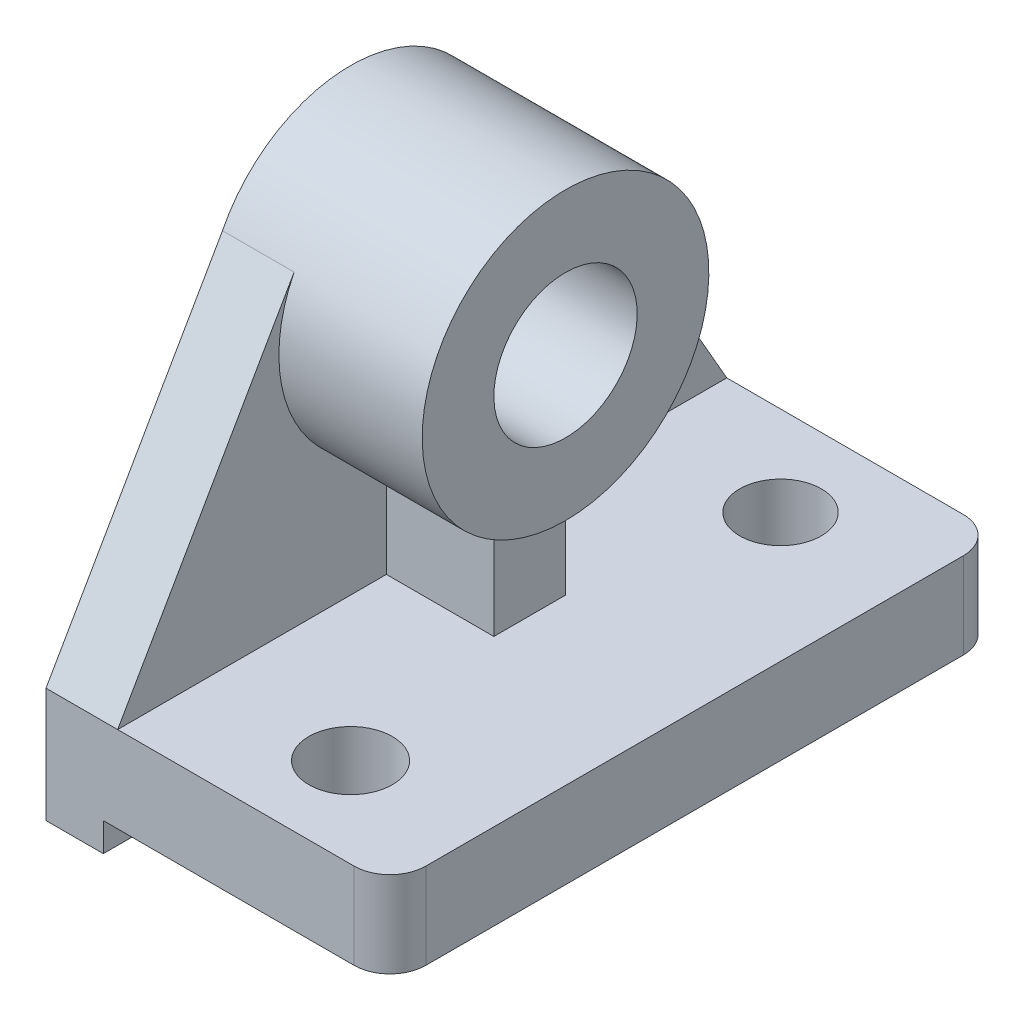
ISO-10303-21;
HEADER;
FILE_DESCRIPTION(('STEP AP214'),'2;1');
FILE_NAME('part.step','',(''),(''),'','','');
FILE_SCHEMA(('AUTOMOTIVE_DESIGN { 1 0 10303 214 1 1 1 1 }'));
ENDSEC;
DATA;
#1=APPLICATION_CONTEXT('core data for automotive mechanical design processes');
#2=APPLICATION_PROTOCOL_DEFINITION('international standard','automotive_design',2000,#1);
#3=PRODUCT_CONTEXT('',#1,'mechanical');
#4=PRODUCT('Part','Part','',(#3));
#5=PRODUCT_RELATED_PRODUCT_CATEGORY('part','',(#4));
#6=PRODUCT_DEFINITION_FORMATION('','',#4);
#7=PRODUCT_DEFINITION_CONTEXT('part definition',#1,'design');
#8=PRODUCT_DEFINITION('design','',#6,#7);
#9=PRODUCT_DEFINITION_SHAPE('','',#8);
#10=(LENGTH_UNIT() NAMED_UNIT(*) SI_UNIT(.MILLI.,.METRE.));
#11=(NAMED_UNIT(*) PLANE_ANGLE_UNIT() SI_UNIT($,.RADIAN.));
#12=(NAMED_UNIT(*) SI_UNIT($,.STERADIAN.) SOLID_ANGLE_UNIT());
#13=UNCERTAINTY_MEASURE_WITH_UNIT(LENGTH_MEASURE(1.E-05),#10,'distance_accuracy_value','');
#14=(GEOMETRIC_REPRESENTATION_CONTEXT(3) GLOBAL_UNCERTAINTY_ASSIGNED_CONTEXT((#13)) GLOBAL_UNIT_ASSIGNED_CONTEXT((#10,
#11,#12)) REPRESENTATION_CONTEXT('',''));
#15=CARTESIAN_POINT('',(0.,0.,0.));
#16=DIRECTION('',(0.,0.,1.));
#17=DIRECTION('',(1.,0.,0.));
#18=AXIS2_PLACEMENT_3D('',#15,#16,#17);
#19=CARTESIAN_POINT('',(0.,16.,85.));
#20=DIRECTION('',(0.,-1.,0.));
#21=DIRECTION('',(1.,0.,0.));
#22=AXIS2_PLACEMENT_3D('',#19,#20,#21);
#23=PLANE('',#22);
#24=CARTESIAN_POINT('',(30.,16.,12.5));
#25=DIRECTION('',(0.,1.,0.));
#26=DIRECTION('',(-1.,0.,0.));
#27=AXIS2_PLACEMENT_3D('',#24,#25,#26);
#28=CIRCLE('',#27,5.6970542524879);
#29=CARTESIAN_POINT('',(24.3029457475121,16.,12.5));
#30=VERTEX_POINT('',#29);
#31=EDGE_CURVE('E251',#30,#30,#28,.T.);
#32=ORIENTED_EDGE('',*,*,#31,.F.);
#33=EDGE_LOOP('',(#32));
#34=FACE_BOUND('',#33,.T.);
#35=CARTESIAN_POINT('',(30.,16.,72.5));
#36=DIRECTION('',(0.,1.,0.));
#37=DIRECTION('',(-1.,0.,0.));
#38=AXIS2_PLACEMENT_3D('',#35,#36,#37);
#39=CIRCLE('',#38,5.82954388626669);
#40=CARTESIAN_POINT('',(24.1704561137333,16.,72.5));
#41=VERTEX_POINT('',#40);
#42=EDGE_CURVE('E314',#41,#41,#39,.T.);
#43=ORIENTED_EDGE('',*,*,#42,.F.);
#44=EDGE_LOOP('',(#43));
#45=FACE_BOUND('',#44,.T.);
#46=DIRECTION('',(0.,0.,-1.));
#47=VECTOR('',#46,1.);
#48=CARTESIAN_POINT('',(48.,16.,85.));
#49=LINE('',#48,#47);
#50=CARTESIAN_POINT('',(48.,16.,80.));
#51=VERTEX_POINT('',#50);
#52=CARTESIAN_POINT('',(48.,16.,5.));
#53=VERTEX_POINT('',#52);
#54=EDGE_CURVE('E238',#51,#53,#49,.T.);
#55=ORIENTED_EDGE('',*,*,#54,.T.);
#56=CARTESIAN_POINT('',(43.,16.,5.));
#57=DIRECTION('',(0.,-1.,0.));
#58=DIRECTION('',(1.,0.,0.));
#59=AXIS2_PLACEMENT_3D('',#56,#57,#58);
#60=CIRCLE('',#59,5.);
#61=CARTESIAN_POINT('',(43.,16.,0.));
#62=VERTEX_POINT('',#61);
#63=EDGE_CURVE('E265',#53,#62,#60,.F.);
#64=ORIENTED_EDGE('',*,*,#63,.T.);
#65=DIRECTION('',(-1.,0.,0.));
#66=VECTOR('',#65,1.);
#67=CARTESIAN_POINT('',(0.,16.,0.));
#68=LINE('',#67,#66);
#69=CARTESIAN_POINT('',(10.,16.,0.));
#70=VERTEX_POINT('',#69);
#71=EDGE_CURVE('E231',#62,#70,#68,.T.);
#72=ORIENTED_EDGE('',*,*,#71,.T.);
#73=DIRECTION('',(0.,0.,1.));
#74=VECTOR('',#73,1.);
#75=CARTESIAN_POINT('',(10.,16.,0.));
#76=LINE('',#75,#74);
#77=CARTESIAN_POINT('',(10.,16.,37.5));
#78=VERTEX_POINT('',#77);
#79=EDGE_CURVE('E182',#70,#78,#76,.T.);
#80=ORIENTED_EDGE('',*,*,#79,.T.);
#81=DIRECTION('',(-1.,0.,0.));
#82=VECTOR('',#81,1.);
#83=CARTESIAN_POINT('',(10.,16.,37.5));
#84=LINE('',#83,#82);
#85=CARTESIAN_POINT('',(25.,16.,37.5));
#86=VERTEX_POINT('',#85);
#87=EDGE_CURVE('E310',#86,#78,#84,.T.);
#88=ORIENTED_EDGE('',*,*,#87,.F.);
#89=DIRECTION('',(0.,0.,-1.));
#90=VECTOR('',#89,1.);
#91=CARTESIAN_POINT('',(25.,16.,37.5));
#92=LINE('',#91,#90);
#93=CARTESIAN_POINT('',(25.,16.,47.5));
#94=VERTEX_POINT('',#93);
#95=EDGE_CURVE('E176',#94,#86,#92,.T.);
#96=ORIENTED_EDGE('',*,*,#95,.F.);
#97=DIRECTION('',(1.,0.,0.));
#98=VECTOR('',#97,1.);
#99=CARTESIAN_POINT('',(10.,16.,47.5));
#100=LINE('',#99,#98);
#101=CARTESIAN_POINT('',(10.,16.,47.5));
#102=VERTEX_POINT('',#101);
#103=EDGE_CURVE('E160',#102,#94,#100,.T.);
#104=ORIENTED_EDGE('',*,*,#103,.F.);
#105=CARTESIAN_POINT('',(10.,16.,85.));
#106=VERTEX_POINT('',#105);
#107=EDGE_CURVE('E175',#102,#106,#76,.T.);
#108=ORIENTED_EDGE('',*,*,#107,.T.);
#109=DIRECTION('',(-1.,0.,0.));
#110=VECTOR('',#109,1.);
#111=CARTESIAN_POINT('',(0.,16.,85.));
#112=LINE('',#111,#110);
#113=CARTESIAN_POINT('',(43.,16.,85.));
#114=VERTEX_POINT('',#113);
#115=EDGE_CURVE('E224',#114,#106,#112,.T.);
#116=ORIENTED_EDGE('',*,*,#115,.F.);
#117=CARTESIAN_POINT('',(43.,16.,80.));
#118=DIRECTION('',(0.,-1.,0.));
#119=DIRECTION('',(1.,0.,0.));
#120=AXIS2_PLACEMENT_3D('',#117,#118,#119);
#121=CIRCLE('',#120,5.);
#122=EDGE_CURVE('E264',#114,#51,#121,.F.);
#123=ORIENTED_EDGE('',*,*,#122,.T.);
#124=EDGE_LOOP('',(#55,#64,#72,#80,#88,#96,#104,#108,#116,#123));
#125=FACE_BOUND('',#124,.T.);
#126=ADVANCED_FACE('F43',(#34,#45,#125),#23,.F.);
#127=CARTESIAN_POINT('',(10.,0.,0.));
#128=DIRECTION('',(-1.,0.,0.));
#129=DIRECTION('',(0.,-1.,0.));
#130=AXIS2_PLACEMENT_3D('',#127,#128,#129);
#131=PLANE('',#130);
#132=DIRECTION('',(0.,-1.,0.));
#133=VECTOR('',#132,1.);
#134=CARTESIAN_POINT('',(9.99999999999999,70.001,37.5));
#135=LINE('',#134,#133);
#136=CARTESIAN_POINT('',(10.,30.6350832689629,37.5));
#137=VERTEX_POINT('',#136);
#138=EDGE_CURVE('E302',#137,#78,#135,.T.);
#139=ORIENTED_EDGE('',*,*,#138,.T.);
#140=ORIENTED_EDGE('',*,*,#79,.F.);
#141=DIRECTION('',(0.,0.867635064006923,0.497201564464255));
#142=VECTOR('',#141,1.);
#143=CARTESIAN_POINT('',(10.,3.95535033129125,-6.90223217933258));
#144=LINE('',#143,#142);
#145=CARTESIAN_POINT('',(10.,58.9731186911772,24.6259086677379));
#146=VERTEX_POINT('',#145);
#147=EDGE_CURVE('E183',#70,#146,#144,.T.);
#148=ORIENTED_EDGE('',*,*,#147,.T.);
#149=CARTESIAN_POINT('',(10.,50.,42.5));
#150=DIRECTION('',(-1.,0.,0.));
#151=DIRECTION('',(0.,-1.,0.));
#152=AXIS2_PLACEMENT_3D('',#149,#150,#151);
#153=CIRCLE('',#152,20.);
#154=EDGE_CURVE('E191',#146,#137,#153,.T.);
#155=ORIENTED_EDGE('',*,*,#154,.T.);
#156=EDGE_LOOP('',(#139,#140,#148,#155));
#157=FACE_BOUND('',#156,.T.);
#158=ADVANCED_FACE('F328',(#157),#131,.F.);
#159=DIRECTION('',(0.,-1.,0.));
#160=VECTOR('',#159,1.);
#161=CARTESIAN_POINT('',(9.99999999999999,70.001,47.5));
#162=LINE('',#161,#160);
#163=CARTESIAN_POINT('',(10.,30.6350832689629,47.5));
#164=VERTEX_POINT('',#163);
#165=EDGE_CURVE('E155',#164,#102,#162,.T.);
#166=ORIENTED_EDGE('',*,*,#165,.F.);
#167=CARTESIAN_POINT('',(10.,58.9731186911774,60.374091332262));
#168=VERTEX_POINT('',#167);
#169=EDGE_CURVE('E194',#164,#168,#153,.T.);
#170=ORIENTED_EDGE('',*,*,#169,.T.);
#171=DIRECTION('',(0.,0.867635064006923,-0.497201564464255));
#172=VECTOR('',#171,1.);
#173=CARTESIAN_POINT('',(10.,40.6234587839956,70.8894335443479));
#174=LINE('',#173,#172);
#175=EDGE_CURVE('E181',#106,#168,#174,.T.);
#176=ORIENTED_EDGE('',*,*,#175,.F.);
#177=ORIENTED_EDGE('',*,*,#107,.F.);
#178=EDGE_LOOP('',(#166,#170,#176,#177));
#179=FACE_BOUND('',#178,.T.);
#180=ADVANCED_FACE('F177',(#179),#131,.F.);
#181=CARTESIAN_POINT('',(30.,50.,42.5));
#182=DIRECTION('',(-1.,0.,0.));
#183=DIRECTION('',(0.,-1.,0.));
#184=AXIS2_PLACEMENT_3D('',#181,#182,#183);
#185=CYLINDRICAL_SURFACE('',#184,20.);
#186=CARTESIAN_POINT('',(30.,50.,42.5));
#187=DIRECTION('',(-1.,0.,0.));
#188=DIRECTION('',(0.,-1.,0.));
#189=AXIS2_PLACEMENT_3D('',#186,#187,#188);
#190=CIRCLE('',#189,20.);
#191=CARTESIAN_POINT('',(30.,30.,42.5));
#192=VERTEX_POINT('',#191);
#193=EDGE_CURVE('E202',#192,#192,#190,.T.);
#194=ORIENTED_EDGE('',*,*,#193,.T.);
#195=EDGE_LOOP('',(#194));
#196=FACE_BOUND('',#195,.T.);
#197=CARTESIAN_POINT('',(25.,50.,42.5));
#198=DIRECTION('',(-1.,0.,0.));
#199=DIRECTION('',(0.,-1.,0.));
#200=AXIS2_PLACEMENT_3D('',#197,#198,#199);
#201=CIRCLE('',#200,20.);
#202=CARTESIAN_POINT('',(25.,30.6350832689629,37.5));
#203=VERTEX_POINT('',#202);
#204=CARTESIAN_POINT('',(25.,30.6350832689629,47.5));
#205=VERTEX_POINT('',#204);
#206=EDGE_CURVE('E298',#203,#205,#201,.T.);
#207=ORIENTED_EDGE('',*,*,#206,.F.);
#208=DIRECTION('',(-1.,0.,0.));
#209=VECTOR('',#208,1.);
#210=CARTESIAN_POINT('',(30.,30.6350832689629,37.5));
#211=LINE('',#210,#209);
#212=EDGE_CURVE('E164',#137,#203,#211,.F.);
#213=ORIENTED_EDGE('',*,*,#212,.F.);
#214=ORIENTED_EDGE('',*,*,#154,.F.);
#215=DIRECTION('',(-1.,0.,0.));
#216=VECTOR('',#215,1.);
#217=CARTESIAN_POINT('',(10.,58.9731186911772,24.6259086677379));
#218=LINE('',#217,#216);
#219=CARTESIAN_POINT('',(0.,58.9731186911772,24.6259086677379));
#220=VERTEX_POINT('',#219);
#221=EDGE_CURVE('E201',#146,#220,#218,.T.);
#222=ORIENTED_EDGE('',*,*,#221,.T.);
#223=CARTESIAN_POINT('',(0.,50.,42.5));
#224=DIRECTION('',(-1.,0.,0.));
#225=DIRECTION('',(0.,-1.,0.));
#226=AXIS2_PLACEMENT_3D('',#223,#224,#225);
#227=CIRCLE('',#226,20.);
#228=CARTESIAN_POINT('',(0.,58.9731186911774,60.374091332262));
#229=VERTEX_POINT('',#228);
#230=EDGE_CURVE('E288',#229,#220,#227,.T.);
#231=ORIENTED_EDGE('',*,*,#230,.F.);
#232=DIRECTION('',(-1.,0.,0.));
#233=VECTOR('',#232,1.);
#234=CARTESIAN_POINT('',(10.,58.9731186911774,60.374091332262));
#235=LINE('',#234,#233);
#236=EDGE_CURVE('E210',#168,#229,#235,.T.);
#237=ORIENTED_EDGE('',*,*,#236,.F.);
#238=ORIENTED_EDGE('',*,*,#169,.F.);
#239=DIRECTION('',(-1.,0.,0.));
#240=VECTOR('',#239,1.);
#241=CARTESIAN_POINT('',(30.,30.6350832689629,47.5));
#242=LINE('',#241,#240);
#243=EDGE_CURVE('E163',#205,#164,#242,.T.);
#244=ORIENTED_EDGE('',*,*,#243,.F.);
#245=EDGE_LOOP('',(#207,#213,#214,#222,#231,#237,#238,#244));
#246=FACE_BOUND('',#245,.T.);
#247=ADVANCED_FACE('F352',(#196,#246),#185,.T.);
#248=CARTESIAN_POINT('',(8.,0.,85.));
#249=DIRECTION('',(0.,1.,0.));
#250=DIRECTION('',(-1.,0.,0.));
#251=AXIS2_PLACEMENT_3D('',#248,#249,#250);
#252=PLANE('',#251);
#253=DIRECTION('',(1.,0.,0.));
#254=VECTOR('',#253,1.);
#255=CARTESIAN_POINT('',(8.,0.,0.));
#256=LINE('',#255,#254);
#257=CARTESIAN_POINT('',(0.,0.,0.));
#258=VERTEX_POINT('',#257);
#259=CARTESIAN_POINT('',(8.,0.,0.));
#260=VERTEX_POINT('',#259);
#261=EDGE_CURVE('E207',#258,#260,#256,.T.);
#262=ORIENTED_EDGE('',*,*,#261,.T.);
#263=DIRECTION('',(0.,0.,-1.));
#264=VECTOR('',#263,1.);
#265=CARTESIAN_POINT('',(8.,0.,85.));
#266=LINE('',#265,#264);
#267=CARTESIAN_POINT('',(8.,0.,85.));
#268=VERTEX_POINT('',#267);
#269=EDGE_CURVE('E246',#268,#260,#266,.T.);
#270=ORIENTED_EDGE('',*,*,#269,.F.);
#271=DIRECTION('',(1.,0.,0.));
#272=VECTOR('',#271,1.);
#273=CARTESIAN_POINT('',(8.,0.,85.));
#274=LINE('',#273,#272);
#275=CARTESIAN_POINT('',(0.,0.,85.));
#276=VERTEX_POINT('',#275);
#277=EDGE_CURVE('E211',#276,#268,#274,.T.);
#278=ORIENTED_EDGE('',*,*,#277,.F.);
#279=DIRECTION('',(0.,0.,-1.));
#280=VECTOR('',#279,1.);
#281=CARTESIAN_POINT('',(0.,0.,85.));
#282=LINE('',#281,#280);
#283=EDGE_CURVE('E228',#276,#258,#282,.T.);
#284=ORIENTED_EDGE('',*,*,#283,.T.);
#285=EDGE_LOOP('',(#262,#270,#278,#284));
#286=FACE_BOUND('',#285,.T.);
#287=ADVANCED_FACE('F348',(#286),#252,.F.);
#288=CARTESIAN_POINT('',(8.,4.,85.));
#289=DIRECTION('',(-1.,0.,0.));
#290=DIRECTION('',(0.,0.,1.));
#291=AXIS2_PLACEMENT_3D('',#288,#289,#290);
#292=PLANE('',#291);
#293=DIRECTION('',(0.,1.,0.));
#294=VECTOR('',#293,1.);
#295=CARTESIAN_POINT('',(8.,4.,0.));
#296=LINE('',#295,#294);
#297=CARTESIAN_POINT('',(8.,4.,0.));
#298=VERTEX_POINT('',#297);
#299=EDGE_CURVE('E230',#260,#298,#296,.T.);
#300=ORIENTED_EDGE('',*,*,#299,.T.);
#301=DIRECTION('',(0.,0.,-1.));
#302=VECTOR('',#301,1.);
#303=CARTESIAN_POINT('',(8.,4.,85.));
#304=LINE('',#303,#302);
#305=CARTESIAN_POINT('',(8.,4.,85.));
#306=VERTEX_POINT('',#305);
#307=EDGE_CURVE('E243',#306,#298,#304,.T.);
#308=ORIENTED_EDGE('',*,*,#307,.F.);
#309=DIRECTION('',(0.,1.,0.));
#310=VECTOR('',#309,1.);
#311=CARTESIAN_POINT('',(8.,4.,85.));
#312=LINE('',#311,#310);
#313=EDGE_CURVE('E219',#268,#306,#312,.T.);
#314=ORIENTED_EDGE('',*,*,#313,.F.);
#315=ORIENTED_EDGE('',*,*,#269,.T.);
#316=EDGE_LOOP('',(#300,#308,#314,#315));
#317=FACE_BOUND('',#316,.T.);
#318=ADVANCED_FACE('F336',(#317),#292,.F.);
#319=CARTESIAN_POINT('',(48.,4.00000000000001,85.));
#320=DIRECTION('',(0.,1.,0.));
#321=DIRECTION('',(-1.,0.,0.));
#322=AXIS2_PLACEMENT_3D('',#319,#320,#321);
#323=PLANE('',#322);
#324=CARTESIAN_POINT('',(30.,4.,12.5));
#325=DIRECTION('',(0.,1.,0.));
#326=DIRECTION('',(-1.,0.,0.));
#327=AXIS2_PLACEMENT_3D('',#324,#325,#326);
#328=CIRCLE('',#327,5.6970542524879);
#329=CARTESIAN_POINT('',(24.3029457475121,4.,12.5));
#330=VERTEX_POINT('',#329);
#331=EDGE_CURVE('E254',#330,#330,#328,.T.);
#332=ORIENTED_EDGE('',*,*,#331,.T.);
#333=EDGE_LOOP('',(#332));
#334=FACE_BOUND('',#333,.T.);
#335=CARTESIAN_POINT('',(30.,4.,72.5));
#336=DIRECTION('',(0.,1.,0.));
#337=DIRECTION('',(-1.,0.,0.));
#338=AXIS2_PLACEMENT_3D('',#335,#336,#337);
#339=CIRCLE('',#338,5.82954388626669);
#340=CARTESIAN_POINT('',(24.1704561137333,4.,72.5));
#341=VERTEX_POINT('',#340);
#342=EDGE_CURVE('E249',#341,#341,#339,.T.);
#343=ORIENTED_EDGE('',*,*,#342,.T.);
#344=EDGE_LOOP('',(#343));
#345=FACE_BOUND('',#344,.T.);
#346=DIRECTION('',(1.,0.,0.));
#347=VECTOR('',#346,1.);
#348=CARTESIAN_POINT('',(48.,4.00000000000001,0.));
#349=LINE('',#348,#347);
#350=CARTESIAN_POINT('',(43.,4.,0.));
#351=VERTEX_POINT('',#350);
#352=EDGE_CURVE('E233',#298,#351,#349,.T.);
#353=ORIENTED_EDGE('',*,*,#352,.T.);
#354=CARTESIAN_POINT('',(43.,4.00000000000001,5.));
#355=DIRECTION('',(0.,1.,0.));
#356=DIRECTION('',(-1.,0.,0.));
#357=AXIS2_PLACEMENT_3D('',#354,#355,#356);
#358=CIRCLE('',#357,5.);
#359=CARTESIAN_POINT('',(48.,4.00000000000001,5.));
#360=VERTEX_POINT('',#359);
#361=EDGE_CURVE('E51',#351,#360,#358,.F.);
#362=ORIENTED_EDGE('',*,*,#361,.T.);
#363=DIRECTION('',(0.,0.,-1.));
#364=VECTOR('',#363,1.);
#365=CARTESIAN_POINT('',(48.,4.00000000000001,85.));
#366=LINE('',#365,#364);
#367=CARTESIAN_POINT('',(48.,4.00000000000001,80.));
#368=VERTEX_POINT('',#367);
#369=EDGE_CURVE('E239',#368,#360,#366,.T.);
#370=ORIENTED_EDGE('',*,*,#369,.F.);
#371=CARTESIAN_POINT('',(43.,4.,80.));
#372=DIRECTION('',(0.,1.,0.));
#373=DIRECTION('',(-1.,0.,0.));
#374=AXIS2_PLACEMENT_3D('',#371,#372,#373);
#375=CIRCLE('',#374,5.);
#376=CARTESIAN_POINT('',(43.,4.,85.));
#377=VERTEX_POINT('',#376);
#378=EDGE_CURVE('E59',#368,#377,#375,.F.);
#379=ORIENTED_EDGE('',*,*,#378,.T.);
#380=DIRECTION('',(1.,0.,0.));
#381=VECTOR('',#380,1.);
#382=CARTESIAN_POINT('',(48.,4.00000000000001,85.));
#383=LINE('',#382,#381);
#384=EDGE_CURVE('E216',#306,#377,#383,.T.);
#385=ORIENTED_EDGE('',*,*,#384,.F.);
#386=ORIENTED_EDGE('',*,*,#307,.T.);
#387=EDGE_LOOP('',(#353,#362,#370,#379,#385,#386));
#388=FACE_BOUND('',#387,.T.);
#389=ADVANCED_FACE('F270',(#334,#345,#388),#323,.F.);
#390=CARTESIAN_POINT('',(48.,16.,85.));
#391=DIRECTION('',(-1.,0.,0.));
#392=DIRECTION('',(0.,0.,1.));
#393=AXIS2_PLACEMENT_3D('',#390,#391,#392);
#394=PLANE('',#393);
#395=ORIENTED_EDGE('',*,*,#369,.T.);
#396=DIRECTION('',(0.,1.,0.));
#397=VECTOR('',#396,1.);
#398=CARTESIAN_POINT('',(48.,16.,5.));
#399=LINE('',#398,#397);
#400=EDGE_CURVE('E256',#360,#53,#399,.T.);
#401=ORIENTED_EDGE('',*,*,#400,.T.);
#402=ORIENTED_EDGE('',*,*,#54,.F.);
#403=DIRECTION('',(0.,1.,0.));
#404=VECTOR('',#403,1.);
#405=CARTESIAN_POINT('',(48.,16.,80.));
#406=LINE('',#405,#404);
#407=EDGE_CURVE('E248',#51,#368,#406,.F.);
#408=ORIENTED_EDGE('',*,*,#407,.T.);
#409=EDGE_LOOP('',(#395,#401,#402,#408));
#410=FACE_BOUND('',#409,.T.);
#411=ADVANCED_FACE('F275',(#410),#394,.F.);
#412=CARTESIAN_POINT('',(0.,0.,85.));
#413=DIRECTION('',(1.,0.,0.));
#414=DIRECTION('',(0.,1.,0.));
#415=AXIS2_PLACEMENT_3D('',#412,#413,#414);
#416=PLANE('',#415);
#417=CARTESIAN_POINT('',(0.,50.,42.5));
#418=DIRECTION('',(1.,0.,0.));
#419=DIRECTION('',(0.,1.,0.));
#420=AXIS2_PLACEMENT_3D('',#417,#418,#419);
#421=CIRCLE('',#420,10.);
#422=CARTESIAN_POINT('',(0.,60.,42.5));
#423=VERTEX_POINT('',#422);
#424=EDGE_CURVE('E180',#423,#423,#421,.T.);
#425=ORIENTED_EDGE('',*,*,#424,.T.);
#426=EDGE_LOOP('',(#425));
#427=FACE_BOUND('',#426,.T.);
#428=DIRECTION('',(0.,-1.,0.));
#429=VECTOR('',#428,1.);
#430=CARTESIAN_POINT('',(0.,0.,0.));
#431=LINE('',#430,#429);
#432=CARTESIAN_POINT('',(0.,16.,0.));
#433=VERTEX_POINT('',#432);
#434=EDGE_CURVE('E217',#433,#258,#431,.T.);
#435=ORIENTED_EDGE('',*,*,#434,.T.);
#436=ORIENTED_EDGE('',*,*,#283,.F.);
#437=DIRECTION('',(0.,-1.,0.));
#438=VECTOR('',#437,1.);
#439=CARTESIAN_POINT('',(0.,0.,85.));
#440=LINE('',#439,#438);
#441=CARTESIAN_POINT('',(0.,16.,85.));
#442=VERTEX_POINT('',#441);
#443=EDGE_CURVE('E221',#442,#276,#440,.T.);
#444=ORIENTED_EDGE('',*,*,#443,.F.);
#445=DIRECTION('',(0.,0.867635064006923,-0.497201564464255));
#446=VECTOR('',#445,1.);
#447=CARTESIAN_POINT('',(0.,40.6234587839956,70.8894335443479));
#448=LINE('',#447,#446);
#449=EDGE_CURVE('E189',#442,#229,#448,.T.);
#450=ORIENTED_EDGE('',*,*,#449,.T.);
#451=ORIENTED_EDGE('',*,*,#230,.T.);
#452=DIRECTION('',(0.,0.867635064006923,0.497201564464255));
#453=VECTOR('',#452,1.);
#454=CARTESIAN_POINT('',(0.,3.95535033129125,-6.90223217933258));
#455=LINE('',#454,#453);
#456=EDGE_CURVE('E197',#433,#220,#455,.T.);
#457=ORIENTED_EDGE('',*,*,#456,.F.);
#458=EDGE_LOOP('',(#435,#436,#444,#450,#451,#457));
#459=FACE_BOUND('',#458,.T.);
#460=ADVANCED_FACE('F290',(#427,#459),#416,.F.);
#461=CARTESIAN_POINT('',(0.,0.,85.));
#462=DIRECTION('',(0.,0.,-1.));
#463=DIRECTION('',(-1.,0.,0.));
#464=AXIS2_PLACEMENT_3D('',#461,#462,#463);
#465=PLANE('',#464);
#466=ORIENTED_EDGE('',*,*,#384,.T.);
#467=DIRECTION('',(0.,1.,0.));
#468=VECTOR('',#467,1.);
#469=CARTESIAN_POINT('',(43.,0.,85.));
#470=LINE('',#469,#468);
#471=EDGE_CURVE('E11',#377,#114,#470,.T.);
#472=ORIENTED_EDGE('',*,*,#471,.T.);
#473=ORIENTED_EDGE('',*,*,#115,.T.);
#474=DIRECTION('',(-1.,0.,0.));
#475=VECTOR('',#474,1.);
#476=CARTESIAN_POINT('',(10.,16.,85.));
#477=LINE('',#476,#475);
#478=EDGE_CURVE('E208',#106,#442,#477,.T.);
#479=ORIENTED_EDGE('',*,*,#478,.T.);
#480=ORIENTED_EDGE('',*,*,#443,.T.);
#481=ORIENTED_EDGE('',*,*,#277,.T.);
#482=ORIENTED_EDGE('',*,*,#313,.T.);
#483=EDGE_LOOP('',(#466,#472,#473,#479,#480,#481,#482));
#484=FACE_BOUND('',#483,.T.);
#485=ADVANCED_FACE('F392',(#484),#465,.F.);
#486=CARTESIAN_POINT('',(0.,0.,0.));
#487=DIRECTION('',(0.,0.,-1.));
#488=DIRECTION('',(-1.,0.,0.));
#489=AXIS2_PLACEMENT_3D('',#486,#487,#488);
#490=PLANE('',#489);
#491=ORIENTED_EDGE('',*,*,#71,.F.);
#492=DIRECTION('',(0.,1.,0.));
#493=VECTOR('',#492,1.);
#494=CARTESIAN_POINT('',(43.,4.00000000000001,0.));
#495=LINE('',#494,#493);
#496=EDGE_CURVE('E68',#62,#351,#495,.F.);
#497=ORIENTED_EDGE('',*,*,#496,.T.);
#498=ORIENTED_EDGE('',*,*,#352,.F.);
#499=ORIENTED_EDGE('',*,*,#299,.F.);
#500=ORIENTED_EDGE('',*,*,#261,.F.);
#501=ORIENTED_EDGE('',*,*,#434,.F.);
#502=DIRECTION('',(-1.,0.,0.));
#503=VECTOR('',#502,1.);
#504=CARTESIAN_POINT('',(10.,16.,0.));
#505=LINE('',#504,#503);
#506=EDGE_CURVE('E199',#70,#433,#505,.T.);
#507=ORIENTED_EDGE('',*,*,#506,.F.);
#508=EDGE_LOOP('',(#491,#497,#498,#499,#500,#501,#507));
#509=FACE_BOUND('',#508,.T.);
#510=ADVANCED_FACE('F279',(#509),#490,.T.);
#511=CARTESIAN_POINT('',(10.,3.95535033129125,-6.90223217933258));
#512=DIRECTION('',(0.,-0.497201564464255,0.867635064006923));
#513=DIRECTION('',(0.,-0.867635064006923,-0.497201564464255));
#514=AXIS2_PLACEMENT_3D('',#511,#512,#513);
#515=PLANE('',#514);
#516=ORIENTED_EDGE('',*,*,#456,.T.);
#517=ORIENTED_EDGE('',*,*,#221,.F.);
#518=ORIENTED_EDGE('',*,*,#147,.F.);
#519=ORIENTED_EDGE('',*,*,#506,.T.);
#520=EDGE_LOOP('',(#516,#517,#518,#519));
#521=FACE_BOUND('',#520,.T.);
#522=ADVANCED_FACE('F282',(#521),#515,.F.);
#523=CARTESIAN_POINT('',(10.,40.6234587839956,70.8894335443479));
#524=DIRECTION('',(0.,0.497201564464255,0.867635064006923));
#525=DIRECTION('',(0.,-0.867635064006923,0.497201564464255));
#526=AXIS2_PLACEMENT_3D('',#523,#524,#525);
#527=PLANE('',#526);
#528=ORIENTED_EDGE('',*,*,#449,.F.);
#529=ORIENTED_EDGE('',*,*,#478,.F.);
#530=ORIENTED_EDGE('',*,*,#175,.T.);
#531=ORIENTED_EDGE('',*,*,#236,.T.);
#532=EDGE_LOOP('',(#528,#529,#530,#531));
#533=FACE_BOUND('',#532,.T.);
#534=ADVANCED_FACE('F379',(#533),#527,.T.);
#535=CARTESIAN_POINT('',(30.,50.,42.5));
#536=DIRECTION('',(-1.,0.,0.));
#537=DIRECTION('',(0.,-1.,0.));
#538=AXIS2_PLACEMENT_3D('',#535,#536,#537);
#539=PLANE('',#538);
#540=CARTESIAN_POINT('',(30.,50.,42.5));
#541=DIRECTION('',(1.,0.,0.));
#542=DIRECTION('',(0.,1.,0.));
#543=AXIS2_PLACEMENT_3D('',#540,#541,#542);
#544=CIRCLE('',#543,10.);
#545=CARTESIAN_POINT('',(30.,60.,42.5));
#546=VERTEX_POINT('',#545);
#547=EDGE_CURVE('E260',#546,#546,#544,.T.);
#548=ORIENTED_EDGE('',*,*,#547,.F.);
#549=EDGE_LOOP('',(#548));
#550=FACE_BOUND('',#549,.T.);
#551=ORIENTED_EDGE('',*,*,#193,.F.);
#552=EDGE_LOOP('',(#551));
#553=FACE_BOUND('',#552,.T.);
#554=ADVANCED_FACE('F371',(#550,#553),#539,.F.);
#555=CARTESIAN_POINT('',(9.99999999999999,70.001,37.5));
#556=DIRECTION('',(0.,0.,1.));
#557=DIRECTION('',(1.,0.,0.));
#558=AXIS2_PLACEMENT_3D('',#555,#556,#557);
#559=PLANE('',#558);
#560=ORIENTED_EDGE('',*,*,#138,.F.);
#561=ORIENTED_EDGE('',*,*,#212,.T.);
#562=DIRECTION('',(0.,-1.,0.));
#563=VECTOR('',#562,1.);
#564=CARTESIAN_POINT('',(25.,70.001,37.5));
#565=LINE('',#564,#563);
#566=EDGE_CURVE('E305',#203,#86,#565,.T.);
#567=ORIENTED_EDGE('',*,*,#566,.T.);
#568=ORIENTED_EDGE('',*,*,#87,.T.);
#569=EDGE_LOOP('',(#560,#561,#567,#568));
#570=FACE_BOUND('',#569,.T.);
#571=ADVANCED_FACE('F370',(#570),#559,.F.);
#572=CARTESIAN_POINT('',(25.,70.001,37.5));
#573=DIRECTION('',(-1.,0.,0.));
#574=DIRECTION('',(0.,-1.,0.));
#575=AXIS2_PLACEMENT_3D('',#572,#573,#574);
#576=PLANE('',#575);
#577=ORIENTED_EDGE('',*,*,#566,.F.);
#578=ORIENTED_EDGE('',*,*,#206,.T.);
#579=DIRECTION('',(0.,-1.,0.));
#580=VECTOR('',#579,1.);
#581=CARTESIAN_POINT('',(25.,70.001,47.5));
#582=LINE('',#581,#580);
#583=EDGE_CURVE('E168',#205,#94,#582,.T.);
#584=ORIENTED_EDGE('',*,*,#583,.T.);
#585=ORIENTED_EDGE('',*,*,#95,.T.);
#586=EDGE_LOOP('',(#577,#578,#584,#585));
#587=FACE_BOUND('',#586,.T.);
#588=ADVANCED_FACE('F369',(#587),#576,.F.);
#589=CARTESIAN_POINT('',(9.99999999999999,70.001,47.5));
#590=DIRECTION('',(0.,0.,-1.));
#591=DIRECTION('',(-1.,0.,0.));
#592=AXIS2_PLACEMENT_3D('',#589,#590,#591);
#593=PLANE('',#592);
#594=ORIENTED_EDGE('',*,*,#583,.F.);
#595=ORIENTED_EDGE('',*,*,#243,.T.);
#596=ORIENTED_EDGE('',*,*,#165,.T.);
#597=ORIENTED_EDGE('',*,*,#103,.T.);
#598=EDGE_LOOP('',(#594,#595,#596,#597));
#599=FACE_BOUND('',#598,.T.);
#600=ADVANCED_FACE('F159',(#599),#593,.F.);
#601=CARTESIAN_POINT('',(0.,50.,42.5));
#602=DIRECTION('',(1.,0.,0.));
#603=DIRECTION('',(0.,1.,0.));
#604=AXIS2_PLACEMENT_3D('',#601,#602,#603);
#605=CYLINDRICAL_SURFACE('',#604,10.);
#606=ORIENTED_EDGE('',*,*,#424,.F.);
#607=EDGE_LOOP('',(#606));
#608=FACE_BOUND('',#607,.T.);
#609=ORIENTED_EDGE('',*,*,#547,.T.);
#610=EDGE_LOOP('',(#609));
#611=FACE_BOUND('',#610,.T.);
#612=ADVANCED_FACE('F335',(#608,#611),#605,.F.);
#613=CARTESIAN_POINT('',(30.,0.,72.5));
#614=DIRECTION('',(0.,1.,0.));
#615=DIRECTION('',(-1.,0.,0.));
#616=AXIS2_PLACEMENT_3D('',#613,#614,#615);
#617=CYLINDRICAL_SURFACE('',#616,5.82954388626669);
#618=ORIENTED_EDGE('',*,*,#42,.T.);
#619=EDGE_LOOP('',(#618));
#620=FACE_BOUND('',#619,.T.);
#621=ORIENTED_EDGE('',*,*,#342,.F.);
#622=EDGE_LOOP('',(#621));
#623=FACE_BOUND('',#622,.T.);
#624=ADVANCED_FACE('F326',(#620,#623),#617,.F.);
#625=CARTESIAN_POINT('',(30.,0.,12.5));
#626=DIRECTION('',(0.,1.,0.));
#627=DIRECTION('',(-1.,0.,0.));
#628=AXIS2_PLACEMENT_3D('',#625,#626,#627);
#629=CYLINDRICAL_SURFACE('',#628,5.6970542524879);
#630=ORIENTED_EDGE('',*,*,#31,.T.);
#631=EDGE_LOOP('',(#630));
#632=FACE_BOUND('',#631,.T.);
#633=ORIENTED_EDGE('',*,*,#331,.F.);
#634=EDGE_LOOP('',(#633));
#635=FACE_BOUND('',#634,.T.);
#636=ADVANCED_FACE('F322',(#632,#635),#629,.F.);
#637=CARTESIAN_POINT('',(43.,16.,5.));
#638=DIRECTION('',(0.,-1.,0.));
#639=DIRECTION('',(0.,0.,-1.));
#640=AXIS2_PLACEMENT_3D('',#637,#638,#639);
#641=CYLINDRICAL_SURFACE('',#640,5.);
#642=ORIENTED_EDGE('',*,*,#361,.F.);
#643=ORIENTED_EDGE('',*,*,#496,.F.);
#644=ORIENTED_EDGE('',*,*,#63,.F.);
#645=ORIENTED_EDGE('',*,*,#400,.F.);
#646=EDGE_LOOP('',(#642,#643,#644,#645));
#647=FACE_BOUND('',#646,.T.);
#648=ADVANCED_FACE('F273',(#647),#641,.T.);
#649=CARTESIAN_POINT('',(43.,0.,80.));
#650=DIRECTION('',(0.,1.,0.));
#651=DIRECTION('',(0.,0.,1.));
#652=AXIS2_PLACEMENT_3D('',#649,#650,#651);
#653=CYLINDRICAL_SURFACE('',#652,5.);
#654=ORIENTED_EDGE('',*,*,#378,.F.);
#655=ORIENTED_EDGE('',*,*,#407,.F.);
#656=ORIENTED_EDGE('',*,*,#122,.F.);
#657=ORIENTED_EDGE('',*,*,#471,.F.);
#658=EDGE_LOOP('',(#654,#655,#656,#657));
#659=FACE_BOUND('',#658,.T.);
#660=ADVANCED_FACE('F44',(#659),#653,.T.);
#661=CLOSED_SHELL('',(#126,#158,#180,#247,#287,#318,#389,#411,#460,#485,#510,#522,#534,#554,
#571,#588,#600,#612,#624,#636,#648,#660));
#662=MANIFOLD_SOLID_BREP('B2',#661);
#663=ADVANCED_BREP_SHAPE_REPRESENTATION('',(#18,#662),#14);
#664=SHAPE_DEFINITION_REPRESENTATION(#9,#663);
ENDSEC;
END-ISO-10303-21;
